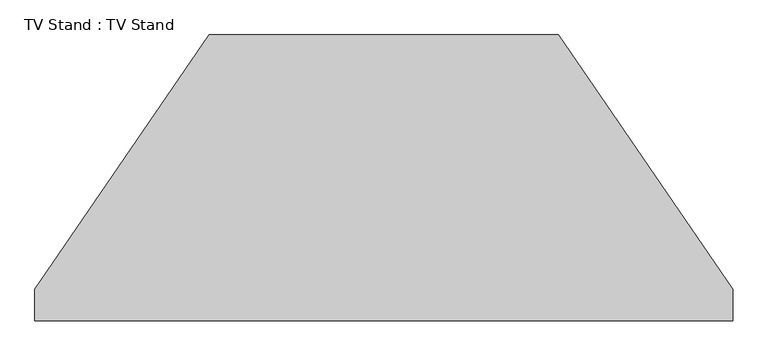
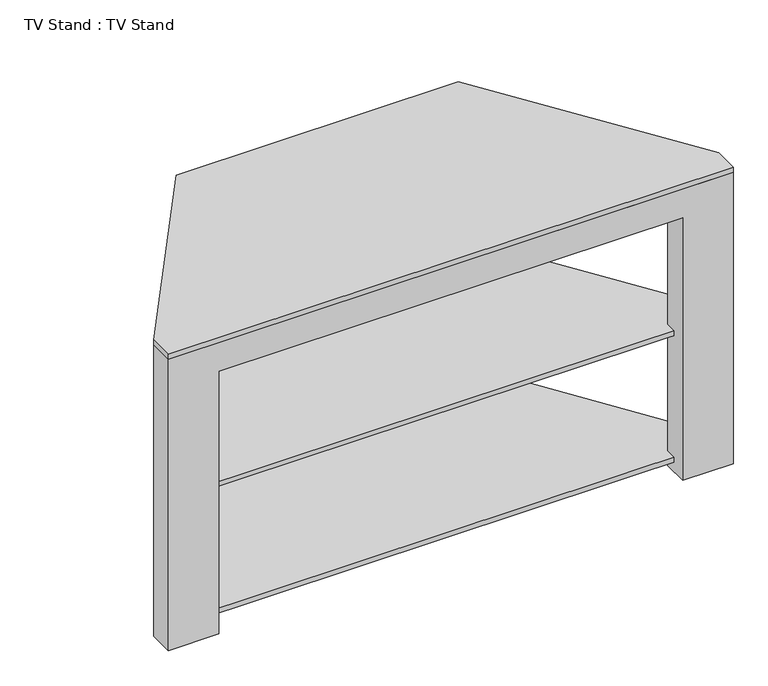
"""IFC4 building model written with IfcOpenShell, lengths in millimetres: furniture geometry, TV Stand : TV Stand."""

from ifc_helpers import new_model, si_unit, point, frame, frame_2d, origin, place, context, project, spatial, polyline, circle_curve, trimmed, segment, composite_curve, outline, extrude, faceted_brep, source, transform, mapped, element, save


def tv_stand_tv_stand_94947415(model_context):
    return source(origin(), model_context, "Body", "SolidModel", [
        extrude(outline(polyline([(425.1724814, -30.0), (633.9880021, -334.3295634), (633.9880021, -427.2), (-383.6119979, -427.2), (-383.6119979, -334.3295634), (-174.7964773, -30.0), (425.1724814, -30.0)])), frame((0.0, 0.0, 20.0), z_axis=(0.0, 0.0, 1.0), x_axis=(1.0, 0.0, 0.0)), (0.0, 0.0, 1.0), 10.0),
        extrude(outline(polyline([(425.1724814, -30.0), (633.9880021, -334.3295634), (633.9880021, -427.2), (-383.6119979, -427.2), (-383.6119979, -334.3295634), (-174.7964773, -30.0), (425.1724814, -30.0)])), frame((0.0, 0.0, 284.8), z_axis=(0.0, 0.0, 1.0), x_axis=(1.0, 0.0, 0.0)), (0.0, 0.0, 1.0), 10.0),
        extrude(outline(polyline([(404.5880021, 0.0), (683.9880021, -407.2), (683.9880021, -457.2), (-433.6119979, -457.2), (-433.6119979, -407.2), (-154.2119979, 0.0), (404.5880021, 0.0)])), frame((0.0, 0.0, 609.6), z_axis=(0.0, 0.0, 1.0), x_axis=(1.0, 0.0, 0.0)), (0.0, 0.0, 1.0), 10.0),
        extrude(outline(polyline([(-50.0, 609.6), (0.0, 609.6), (0.0, 0.0), (-50.0, 0.0), (-50.0, 20.0), (-30.0, 20.0), (-30.0, 30.0), (-50.0, 30.0), (-50.0, 284.8), (-30.0, 284.8), (-30.0, 294.8), (-50.0, 294.8), (-50.0, 609.6)])), frame((-154.2119979, 0.0, 0.0), z_axis=(1.0, 0.0, 0.0), x_axis=(0.0, 1.0, 0.0)), (0.0, 0.0, 1.0), 100.0),
        extrude(outline(polyline([(-50.0, 609.6), (0.0, 609.6), (0.0, 0.0), (-50.0, 0.0), (-50.0, 20.0), (-30.0, 20.0), (-30.0, 30.0), (-50.0, 30.0), (-50.0, 284.8), (-30.0, 284.8), (-30.0, 294.8), (-50.0, 294.8), (-50.0, 609.6)])), frame((304.5880021, 0.0, 0.0), z_axis=(1.0, 0.0, 0.0), x_axis=(0.0, 1.0, 0.0)), (0.0, 0.0, 1.0), 100.0),
        faceted_brep([(-433.6119979, -457.2, 0.0), (-333.6119979, -457.2, 0.0), (-333.6119979, -457.2, 549.6), (583.9880021, -457.2, 549.6), (583.9880021, -457.2, 0.0), (683.9880021, -457.2, 0.0), (683.9880021, -457.2, 609.6), (-433.6119979, -457.2, 609.6), (-433.6119979, -407.2, 0.0), (-433.6119979, -407.2, 609.6), (683.9880021, -407.2, 609.6), (683.9880021, -407.2, 0.0), (583.9880021, -407.2, 0.0), (583.9880021, -407.2, 20.0), (633.9880021, -407.2, 20.0), (633.9880021, -407.2, 30.0), (583.9880021, -407.2, 30.0), (583.9880021, -407.2, 284.8), (633.9880021, -407.2, 284.8), (633.9880021, -407.2, 294.8), (583.9880021, -407.2, 294.8), (583.9880021, -407.2, 549.6), (-333.6119979, -407.2, 549.6), (-333.6119979, -407.2, 294.8), (-383.6119979, -407.2, 294.8), (-383.6119979, -407.2, 284.8), (-333.6119979, -407.2, 284.8), (-333.6119979, -407.2, 30.0), (-383.6119979, -407.2, 30.0), (-383.6119979, -407.2, 20.0), (-333.6119979, -407.2, 20.0), (-333.6119979, -407.2, 0.0), (-333.6119979, -427.2, 20.0), (-333.6119979, -427.2, 30.0), (-333.6119979, -427.2, 284.8), (-333.6119979, -427.2, 294.8), (583.9880021, -427.2, 294.8), (583.9880021, -427.2, 284.8), (583.9880021, -427.2, 30.0), (583.9880021, -427.2, 20.0), (633.9880021, -427.2, 294.8), (-383.6119979, -427.2, 294.8), (-383.6119979, -427.2, 284.8), (633.9880021, -427.2, 284.8), (633.9880021, -427.2, 30.0), (-383.6119979, -427.2, 30.0), (-383.6119979, -427.2, 20.0), (633.9880021, -427.2, 20.0)], [[[0, 1, 2, 3, 4, 5, 6, 7]], [[8, 9, 10, 11, 12, 13, 14, 15, 16, 17, 18, 19, 20, 21, 22, 23, 24, 25, 26, 27, 28, 29, 30, 31]], [[1, 0, 8, 31]], [[2, 1, 31, 30, 32, 33, 27, 26, 34, 35, 23, 22]], [[3, 2, 22, 21]], [[4, 3, 21, 20, 36, 37, 17, 16, 38, 39, 13, 12]], [[5, 4, 12, 11]], [[6, 5, 11, 10]], [[7, 6, 10, 9]], [[0, 7, 9, 8]], [[19, 40, 36, 20]], [[35, 41, 24, 23]], [[25, 42, 34, 26]], [[37, 43, 18, 17]], [[41, 42, 25, 24]], [[42, 41, 35, 34]], [[40, 43, 37, 36]], [[43, 40, 19, 18]], [[15, 44, 38, 16]], [[33, 45, 28, 27]], [[29, 46, 32, 30]], [[39, 47, 14, 13]], [[45, 46, 29, 28]], [[46, 45, 33, 32]], [[44, 47, 39, 38]], [[47, 44, 15, 14]]]),
        extrude(outline(polyline([(0.0, 304.5880021), (609.6, 304.5880021), (609.6, -54.2119979), (0.0, -54.2119979), (0.0, 304.5880021)]), holes=[composite_curve([segment(polyline([(299.8, 145.1700818), (299.8, 105.2059224)]), True, "CONTINUOUS"), segment(trimmed(circle_curve(frame_2d((312.3, 105.2059224)), 12.5), [point((299.8, 105.2059224))], [point((324.8, 105.2059224))], True, "CARTESIAN"), True, "CONTINUOUS"), segment(polyline([(324.8, 105.2059224), (324.8, 145.1700818)]), True, "CONTINUOUS"), segment(trimmed(circle_curve(frame_2d((312.3, 145.1700818)), 12.5), [point((324.8, 145.1700818))], [point((299.8, 145.1700818))], True, "CARTESIAN"), True, "CONTINUOUS")], self_intersect=False), composite_curve([segment(polyline([(35.0, 145.1880021), (35.0, 105.2059224)]), True, "CONTINUOUS"), segment(trimmed(circle_curve(frame_2d((47.5, 105.2059224)), 12.5), [point((35.0, 105.2059224))], [point((60.0, 105.2059224))], True, "CARTESIAN"), True, "CONTINUOUS"), segment(polyline([(60.0, 105.2059224), (60.0, 145.1880021)]), True, "CONTINUOUS"), segment(trimmed(circle_curve(frame_2d((47.5, 145.1880021)), 12.5), [point((60.0, 145.1880021))], [point((35.0, 145.1880021))], True, "CARTESIAN"), True, "CONTINUOUS")], self_intersect=False)]), frame((0.0, -30.0, 0.0), z_axis=(0.0, 1.0, 0.0), x_axis=(0.0, 0.0, 1.0)), (0.0, 0.0, 1.0), 10.0),
    ])


if __name__ == "__main__":
    model = new_model("IFC4")
    model_context = context("Model", 3, world=origin())
    ifc_project = project(units=[si_unit("LENGTHUNIT", "METRE", prefix="MILLI")], contexts=[model_context])
    site = spatial("IfcSite", under=ifc_project)
    building = spatial("IfcBuilding", under=site)
    placement = place(None, origin())
    tv_stand_tv_stand_shape = tv_stand_tv_stand_94947415(model_context)
    element("IfcFurniture", 1, ObjectType="TV Stand : TV Stand", at=placement, inside=building, context=model_context, shape_type="MappedRepresentation", body=[
        mapped(tv_stand_tv_stand_shape, transform((0.0, 0.0, 0.0), x_axis=(1.0, 0.0, 0.0), y_axis=(0.0, 1.0, 0.0), z_axis=(0.0, 0.0, 1.0))),
    ])
    save(model, "model.ifc")

# Revit data of these elements
# Type "TV Stand : TV Stand"
#   Depth = 1' - 6"
#   Width = 3' - 8"
#   Height = 2' - 0"
#   Finish = Melamine - Gray
#   Default Elevation = 0
# Element 1 (IfcFurniture, "TV Stand : TV Stand")
#   Materials on its faces: "Melamine - Gray", "Glass - Shelves"
# Materials
#   "Melamine - Gray": class "Wood", colour RGB 49 49 49, transparency 0
#   "Glass - Shelves": class "Glass", colour RGB 167 167 167, transparency 0.9
